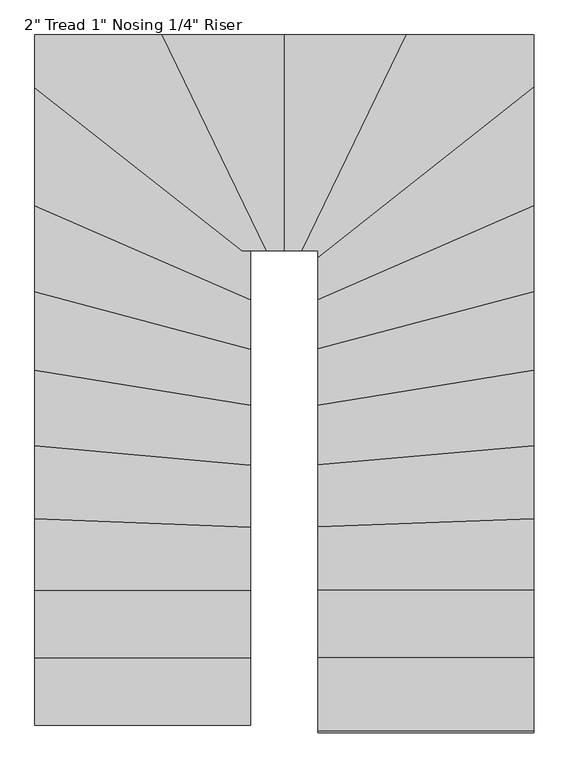
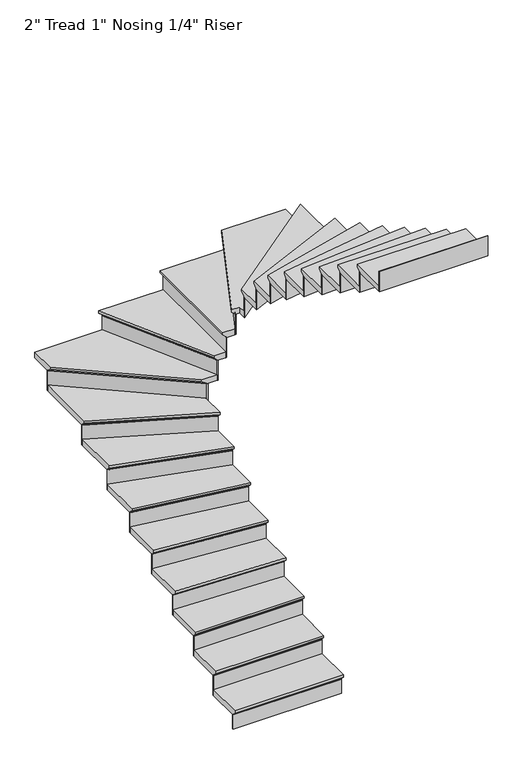
"""IFC4 building model written with IfcOpenShell, lengths in millimetres: stair flight geometry."""

from ifc_helpers import new_model, si_unit, origin, place, context, project, spatial, faceted_brep, source, transform, mapped, element, save


def stair_flight_d4b8cc4c(model_context):
    return source(origin(), model_context, "Body", "Brep", [
        faceted_brep([(-5047.1987704, -4554.2130548, 40388.7214286), (-5047.1987704, -4554.2130548, 40407.7714286), (-5940.8822214, -4554.2130548, 40407.7714286), (-5940.8822214, -4554.2130548, 40388.7214286), (-5047.1987704, -4528.8130548, 40363.3214286), (-5940.8822214, -4528.8130548, 40363.3214286), (-5047.1987704, -4249.4130548, 40407.7714286), (-5940.8822214, -4249.4130548, 40407.7714286), (-5940.8822214, -4528.8130548, 40356.9714286), (-5940.8822214, -4249.4130548, 40356.9714286), (-5047.1987704, -4249.4130548, 40356.9714286), (-5047.1987704, -4528.8130548, 40356.9714286)], [[[0, 1, 2, 3]], [[4, 0, 3, 5]], [[2, 1, 6, 7]], [[8, 9, 10, 11]], [[2, 7, 9, 8, 5, 3]], [[8, 11, 4, 5]], [[6, 1, 0, 4, 11, 10]], [[7, 6, 10, 9]]]),
        faceted_brep([(-5047.1987704, -4528.8130548, 40356.9714286), (-5047.1987704, -4528.8130548, 40233.6), (-5047.1987704, -4522.4630548, 40233.6), (-5047.1987704, -4522.4630548, 40356.9714286), (-5940.8822214, -4528.8130548, 40356.9714286), (-5940.8822214, -4522.4630548, 40356.9714286), (-5940.8822214, -4522.4630548, 40233.6), (-5940.8822214, -4528.8130548, 40233.6)], [[[0, 1, 2, 3]], [[4, 5, 6, 7]], [[1, 0, 4, 7]], [[2, 1, 7, 6]], [[3, 2, 6, 5]], [[0, 3, 5, 4]]]),
        faceted_brep([(-5047.1987704, -4249.4130548, 40531.1428571), (-5047.1987704, -4249.4130548, 40356.9714286), (-5047.1987704, -4243.0630548, 40356.9714286), (-5047.1987704, -4243.0630548, 40531.1428571), (-5940.8822214, -4249.4130548, 40531.1428571), (-5940.8822214, -4243.0630548, 40531.1428571), (-5940.8822214, -4243.0630548, 40356.9714286), (-5940.8822214, -4249.4130548, 40356.9714286)], [[[0, 1, 2, 3]], [[4, 5, 6, 7]], [[1, 0, 4, 7]], [[2, 1, 7, 6]], [[3, 2, 6, 5]], [[0, 3, 5, 4]]]),
        faceted_brep([(-5940.8822214, -4274.8130548, 40581.9428571), (-5047.1987704, -4274.8130548, 40581.9428571), (-5047.1987704, -3970.0130548, 40581.9428571), (-5940.8822214, -3970.0130548, 40581.9428571), (-5940.8822214, -4249.4130548, 40531.1428571), (-5940.8822214, -3970.0130548, 40531.1428571), (-5047.1987704, -3970.0130548, 40531.1428571), (-5047.1987704, -4249.4130548, 40531.1428571), (-5940.8822214, -4249.4130548, 40537.4928571), (-5940.8822214, -4274.8130548, 40562.8928571), (-5047.1987704, -4249.4130548, 40537.4928571), (-5047.1987704, -4274.8130548, 40562.8928571)], [[[0, 1, 2, 3]], [[4, 5, 6, 7]], [[0, 3, 5, 4, 8, 9]], [[4, 7, 10, 8]], [[2, 1, 11, 10, 7, 6]], [[3, 2, 6, 5]], [[11, 1, 0, 9]], [[10, 11, 9, 8]]]),
        faceted_brep([(-5047.1987704, -3970.0130548, 40705.3142857), (-5047.1987704, -3970.0130548, 40531.1428571), (-5047.1987704, -3963.6630548, 40531.1428571), (-5047.1987704, -3963.6630548, 40705.3142857), (-5940.8822214, -3970.0130548, 40705.3142857), (-5940.8822214, -3963.6630548, 40705.3142857), (-5940.8822214, -3963.6630548, 40531.1428571), (-5940.8822214, -3970.0130548, 40531.1428571)], [[[0, 1, 2, 3]], [[4, 5, 6, 7]], [[1, 0, 4, 7]], [[2, 1, 7, 6]], [[3, 2, 6, 5]], [[0, 3, 5, 4]]]),
        faceted_brep([(-5940.8822214, -3995.4130548, 40756.1142857), (-5047.1987704, -3995.4130548, 40756.1142857), (-5047.1987704, -3707.9036879, 40756.1142857), (-5940.8822214, -3673.2843203, 40756.1142857), (-5940.8822214, -3970.0130548, 40705.3142857), (-5940.8822214, -3673.2843203, 40705.3142857), (-5047.1987704, -3707.9036879, 40705.3142857), (-5047.1987704, -3970.0130548, 40705.3142857), (-5940.8822214, -3970.0130548, 40711.6642857), (-5940.8822214, -3995.4130548, 40737.0642857), (-5047.1987704, -3970.0130548, 40711.6642857), (-5047.1987704, -3995.4130548, 40737.0642857)], [[[0, 1, 2, 3]], [[4, 5, 6, 7]], [[0, 3, 5, 4, 8, 9]], [[4, 7, 10, 8]], [[2, 1, 11, 10, 7, 6]], [[3, 2, 6, 5]], [[11, 1, 0, 9]], [[10, 11, 9, 8]]]),
        faceted_brep([(-5047.1987704, -3707.9036879, 40879.4857143), (-5047.1987704, -3707.9036879, 40705.3142857), (-5047.1987704, -3701.5489252, 40705.3142857), (-5047.1987704, -3701.5489252, 40879.4857143), (-5940.8822214, -3673.2843203, 40879.4857143), (-5940.8822214, -3666.9295576, 40879.4857143), (-5940.8822214, -3666.9295576, 40705.3142857), (-5940.8822214, -3673.2843203, 40705.3142857)], [[[0, 1, 2, 3]], [[4, 5, 6, 7]], [[1, 0, 4, 7]], [[2, 1, 7, 6]], [[3, 2, 6, 5]], [[0, 3, 5, 4]]]),
        faceted_brep([(-5940.8822214, -3698.703371, 40930.2857143), (-5047.1987704, -3733.3227386, 40930.2857143), (-5047.1987704, -3451.3234819, 40930.2857143), (-5940.8822214, -3370.89733, 40930.2857143), (-5940.8822214, -3673.2843203, 40879.4857143), (-5940.8822214, -3370.89733, 40879.4857143), (-5047.1987704, -3451.3234819, 40879.4857143), (-5047.1987704, -3707.9036879, 40879.4857143), (-5940.8822214, -3673.2843203, 40885.8357143), (-5940.8822214, -3698.703371, 40911.2357143), (-5047.1987704, -3707.9036879, 40885.8357143), (-5047.1987704, -3733.3227386, 40911.2357143)], [[[0, 1, 2, 3]], [[4, 5, 6, 7]], [[0, 3, 5, 4, 8, 9]], [[4, 7, 10, 8]], [[2, 1, 11, 10, 7, 6]], [[3, 2, 6, 5]], [[11, 1, 0, 9]], [[10, 11, 9, 8]]]),
        faceted_brep([(-5047.1987704, -3451.3234819, 41053.6571429), (-5047.1987704, -3451.3234819, 40879.4857143), (-5047.1987704, -3444.9478197, 40879.4857143), (-5047.1987704, -3444.9478197, 41053.6571429), (-5940.8822214, -3370.89733, 41053.6571429), (-5940.8822214, -3364.5216678, 41053.6571429), (-5940.8822214, -3364.5216678, 40879.4857143), (-5940.8822214, -3370.89733, 40879.4857143)], [[[0, 1, 2, 3]], [[4, 5, 6, 7]], [[1, 0, 4, 7]], [[2, 1, 7, 6]], [[3, 2, 6, 5]], [[0, 3, 5, 4]]]),
        faceted_brep([(-5940.8822214, -3396.3999789, 41104.4571429), (-5047.1987704, -3476.8261308, 41104.4571429), (-5047.1987704, -3203.4301079, 41104.4571429), (-5940.8822214, -3059.5417727, 41104.4571429), (-5940.8822214, -3370.89733, 41053.6571429), (-5940.8822214, -3059.5417727, 41053.6571429), (-5047.1987704, -3203.4301079, 41053.6571429), (-5047.1987704, -3451.3234819, 41053.6571429), (-5940.8822214, -3370.89733, 41060.0071429), (-5940.8822214, -3396.3999789, 41085.4071429), (-5047.1987704, -3451.3234819, 41060.0071429), (-5047.1987704, -3476.8261308, 41085.4071429)], [[[0, 1, 2, 3]], [[4, 5, 6, 7]], [[0, 3, 5, 4, 8, 9]], [[4, 7, 10, 8]], [[2, 1, 11, 10, 7, 6]], [[3, 2, 6, 5]], [[11, 1, 0, 9]], [[10, 11, 9, 8]]]),
        faceted_brep([(-5047.1987704, -3203.4301079, 41227.8285714), (-5047.1987704, -3203.4301079, 41053.6571429), (-5047.1987704, -3196.9983292, 41053.6571429), (-5047.1987704, -3196.9983292, 41227.8285714), (-5940.8822214, -3059.5417727, 41227.8285714), (-5940.8822214, -3053.109994, 41227.8285714), (-5940.8822214, -3053.109994, 41053.6571429), (-5940.8822214, -3059.5417727, 41053.6571429)], [[[0, 1, 2, 3]], [[4, 5, 6, 7]], [[1, 0, 4, 7]], [[2, 1, 7, 6]], [[3, 2, 6, 5]], [[0, 3, 5, 4]]]),
        faceted_brep([(-5940.8822214, -3085.2688872, 41278.6285714), (-5047.1987704, -3229.1572224, 41278.6285714), (-5047.1987704, -2970.3553609, 41278.6285714), (-5940.8822214, -2732.7052783, 41278.6285714), (-5940.8822214, -3059.5417727, 41227.8285714), (-5940.8822214, -2732.7052783, 41227.8285714), (-5047.1987704, -2970.3553609, 41227.8285714), (-5047.1987704, -3203.4301079, 41227.8285714), (-5940.8822214, -3059.5417727, 41234.1785714), (-5940.8822214, -3085.2688872, 41259.5785714), (-5047.1987704, -3203.4301079, 41234.1785714), (-5047.1987704, -3229.1572224, 41259.5785714)], [[[0, 1, 2, 3]], [[4, 5, 6, 7]], [[0, 3, 5, 4, 8, 9]], [[4, 7, 10, 8]], [[2, 1, 11, 10, 7, 6]], [[3, 2, 6, 5]], [[11, 1, 0, 9]], [[10, 11, 9, 8]]]),
        faceted_brep([(-5047.1987704, -2970.3553609, 41402.0), (-5047.1987704, -2970.3553609, 41227.8285714), (-5047.1987704, -2963.7846771, 41227.8285714), (-5047.1987704, -2963.7846771, 41402.0), (-5940.8822214, -2732.7052783, 41402.0), (-5940.8822214, -2726.1345945, 41402.0), (-5940.8822214, -2726.1345945, 41227.8285714), (-5940.8822214, -2732.7052783, 41227.8285714)], [[[0, 1, 2, 3]], [[4, 5, 6, 7]], [[1, 0, 4, 7]], [[2, 1, 7, 6]], [[3, 2, 6, 5]], [[0, 3, 5, 4]]]),
        faceted_brep([(-5940.8822214, -2758.9880136, 41452.8), (-5047.1987704, -2996.6380961, 41452.8), (-5047.1987704, -2765.8050203, 41452.8), (-5940.8822214, -2375.5896532, 41452.8), (-5940.8822214, -2732.7052783, 41402.0), (-5940.8822214, -2375.5896532, 41402.0), (-5047.1987704, -2765.8050203, 41402.0), (-5047.1987704, -2970.3553609, 41402.0), (-5940.8822214, -2732.7052783, 41408.35), (-5940.8822214, -2758.9880136, 41433.75), (-5047.1987704, -2970.3553609, 41408.35), (-5047.1987704, -2996.6380961, 41433.75)], [[[0, 1, 2, 3]], [[4, 5, 6, 7]], [[0, 3, 5, 4, 8, 9]], [[4, 7, 10, 8]], [[2, 1, 11, 10, 7, 6]], [[3, 2, 6, 5]], [[11, 1, 0, 9]], [[10, 11, 9, 8]]]),
        faceted_brep([(-5047.1987704, -2765.8050203, 41576.1714286), (-5047.1987704, -2765.8050203, 41402.0), (-5047.1987704, -2758.8760908, 41402.0), (-5047.1987704, -2758.8760908, 41576.1714286), (-5940.8822214, -2375.5896532, 41576.1714286), (-5940.8822214, -2368.6607237, 41576.1714286), (-5940.8822214, -2368.6607237, 41402.0), (-5940.8822214, -2375.5896532, 41402.0)], [[[0, 1, 2, 3]], [[4, 5, 6, 7]], [[1, 0, 4, 7]], [[2, 1, 7, 6]], [[3, 2, 6, 5]], [[0, 3, 5, 4]]]),
        faceted_brep([(-5940.8822214, -2403.3053713, 41626.9714286), (-5047.1987704, -2793.5207384, 41626.9714286), (-5047.1987704, -2590.8424524, 41626.9714286), (-5040.8038639, -2590.8424524, 41626.9714286), (-5940.8822214, -1882.1944717, 41626.9714286), (-5940.8822214, -2375.5896532, 41576.1714286), (-5940.8822214, -1882.1944717, 41576.1714286), (-5040.8038639, -2590.8424524, 41576.1714286), (-5047.1987704, -2590.8424524, 41576.1714286), (-5047.1987704, -2765.8050203, 41576.1714286), (-5940.8822214, -2375.5896532, 41582.5214286), (-5940.8822214, -2403.3053713, 41607.9214286), (-5047.1987704, -2765.8050203, 41582.5214286), (-5047.1987704, -2793.5207384, 41607.9214286)], [[[0, 1, 2, 3, 4]], [[5, 6, 7, 8, 9]], [[0, 4, 6, 5, 10, 11]], [[5, 9, 12, 10]], [[2, 1, 13, 12, 9, 8]], [[4, 3, 7, 6]], [[13, 1, 0, 11]], [[12, 13, 11, 10]], [[3, 2, 8, 7]]]),
        faceted_brep([(-5040.8038639, -2590.8424524, 41750.3428571), (-5040.8038639, -2590.8424524, 41576.1714286), (-5030.5387554, -2590.8424524, 41576.1714286), (-5030.5387554, -2590.8424524, 41750.3428571), (-5940.8822214, -1882.1944717, 41750.3428571), (-5940.8822214, -1874.1125661, 41750.3428571), (-5940.8822214, -1874.1125661, 41576.1714286), (-5940.8822214, -1882.1944717, 41576.1714286)], [[[0, 1, 2, 3]], [[4, 5, 6, 7]], [[1, 0, 4, 7]], [[2, 1, 7, 6]], [[3, 2, 6, 5]], [[0, 3, 5, 4]]]),
        faceted_brep([(-5384.6489457, -1697.1590014, 41801.1428571), (-5940.8822214, -1697.1590014, 41801.1428571), (-5940.8822214, -1914.5220945, 41801.1428571), (-5081.8642978, -2590.8424524, 41801.1428571), (-4952.3566185, -2590.8424524, 41801.1428571), (-5940.8822214, -1697.1590014, 41750.3428571), (-5384.6489457, -1697.1590014, 41750.3428571), (-4952.3566185, -2590.8424524, 41750.3428571), (-5040.8038639, -2590.8424524, 41750.3428571), (-5940.8822214, -1882.1944717, 41750.3428571), (-5940.8822214, -1882.1944717, 41756.6928571), (-5940.8822214, -1914.5220945, 41782.0928571), (-5040.8038639, -2590.8424524, 41756.6928571), (-5081.8642978, -2590.8424524, 41782.0928571)], [[[0, 1, 2, 3, 4]], [[5, 6, 7, 8, 9]], [[1, 0, 6, 5]], [[2, 1, 5, 9, 10, 11]], [[9, 8, 12, 10]], [[4, 3, 13, 12, 8, 7]], [[0, 4, 7, 6]], [[13, 3, 2, 11]], [[12, 13, 11, 10]]]),
        faceted_brep([(-4952.3566185, -2590.8424524, 41924.5142857), (-4952.3566185, -2590.8424524, 41750.3428571), (-4945.3027294, -2590.8424524, 41750.3428571), (-4945.3027294, -2590.8424524, 41924.5142857), (-5384.6489457, -1697.1590014, 41924.5142857), (-5377.5950566, -1697.1590014, 41924.5142857), (-5377.5950566, -1697.1590014, 41750.3428571), (-5384.6489457, -1697.1590014, 41750.3428571)], [[[0, 1, 2, 3]], [[4, 5, 6, 7]], [[1, 0, 4, 7]], [[2, 1, 7, 6]], [[3, 2, 6, 5]], [[0, 3, 5, 4]]]),
        faceted_brep([(-5412.8645022, -1697.1590014, 41975.3142857), (-4980.5721749, -2590.8424524, 41975.3142857), (-4882.0987704, -2590.8424524, 41975.3142857), (-4882.0987706, -1697.1590014, 41975.3142857), (-5384.6489457, -1697.1590014, 41924.5142857), (-4882.0987706, -1697.1590014, 41924.5142857), (-4882.0987704, -2590.8424524, 41924.5142857), (-4952.3566185, -2590.8424524, 41924.5142857), (-5384.6489457, -1697.1590014, 41930.8642857), (-5412.8645022, -1697.1590014, 41956.2642857), (-4952.3566185, -2590.8424524, 41930.8642857), (-4980.5721749, -2590.8424524, 41956.2642857)], [[[0, 1, 2, 3]], [[4, 5, 6, 7]], [[0, 3, 5, 4, 8, 9]], [[4, 7, 10, 8]], [[3, 2, 6, 5]], [[11, 1, 0, 9]], [[10, 11, 9, 8]], [[2, 1, 11, 10, 7, 6]]]),
        faceted_brep([(-4882.0987704, -2590.8424524, 42098.6857143), (-4882.0987704, -2590.8424524, 41924.5142857), (-4875.7487704, -2590.8424524, 41924.5142857), (-4875.7487704, -2590.8424524, 42098.6857143), (-4882.0987706, -1697.1590014, 42098.6857143), (-4875.7487706, -1697.1590014, 42098.6857143), (-4875.7487706, -1697.1590014, 41924.5142857), (-4882.0987706, -1697.1590014, 41924.5142857)], [[[0, 1, 2, 3]], [[4, 5, 6, 7]], [[1, 0, 4, 7]], [[2, 1, 7, 6]], [[3, 2, 6, 5]], [[0, 3, 5, 4]]]),
        faceted_brep([(-4907.4987706, -1697.1590014, 42149.4857143), (-4907.4987704, -2590.8424524, 42149.4857143), (-4806.2098095, -2590.8424524, 42149.4857143), (-4373.9174828, -1697.1590014, 42149.4857143), (-4882.0987706, -1697.1590014, 42098.6857143), (-4373.9174828, -1697.1590014, 42098.6857143), (-4806.2098095, -2590.8424524, 42098.6857143), (-4882.0987704, -2590.8424524, 42098.6857143), (-4882.0987706, -1697.1590014, 42105.0357143), (-4907.4987706, -1697.1590014, 42130.4357143), (-4882.0987704, -2590.8424524, 42105.0357143), (-4907.4987704, -2590.8424524, 42130.4357143)], [[[0, 1, 2, 3]], [[4, 5, 6, 7]], [[0, 3, 5, 4, 8, 9]], [[4, 7, 10, 8]], [[2, 1, 11, 10, 7, 6]], [[3, 2, 6, 5]], [[11, 1, 0, 9]], [[10, 11, 9, 8]]]),
        faceted_brep([(-4806.2098095, -2590.8424524, 42272.8571429), (-4806.2098095, -2590.8424524, 42098.6857143), (-4799.1559204, -2590.8424524, 42098.6857143), (-4799.1559204, -2590.8424524, 42272.8571429), (-4373.9174828, -1697.1590014, 42272.8571429), (-4366.8635937, -1697.1590014, 42272.8571429), (-4366.8635937, -1697.1590014, 42098.6857143), (-4373.9174828, -1697.1590014, 42098.6857143)], [[[0, 1, 2, 3]], [[4, 5, 6, 7]], [[1, 0, 4, 7]], [[2, 1, 7, 6]], [[3, 2, 6, 5]], [[0, 3, 5, 4]]]),
        faceted_brep([(-3874.1153195, -1946.8497166, 42323.6571429), (-3874.1153195, -1697.1590014, 42323.6571429), (-4402.1330392, -1697.1590014, 42323.6571429), (-4834.4253659, -2590.8424524, 42323.6571429), (-4767.7987704, -2590.8424524, 42323.6571429), (-4767.7987704, -2650.4628721, 42323.6571429), (-3874.1153195, -1697.1590014, 42272.8571429), (-3874.1153195, -1946.8497166, 42272.8571429), (-4767.7987704, -2650.4628721, 42272.8571429), (-4767.7987704, -2590.8424524, 42272.8571429), (-4806.2098095, -2590.8424524, 42272.8571429), (-4373.9174828, -1697.1590014, 42272.8571429), (-4806.2098095, -2590.8424524, 42279.2071429), (-4373.9174828, -1697.1590014, 42279.2071429), (-4834.4253659, -2590.8424524, 42304.6071429), (-4402.1330392, -1697.1590014, 42304.6071429)], [[[0, 1, 2, 3, 4, 5]], [[6, 7, 8, 9, 10, 11]], [[1, 0, 7, 6]], [[11, 10, 12, 13]], [[4, 3, 14, 12, 10, 9]], [[5, 4, 9, 8]], [[0, 5, 8, 7]], [[14, 3, 2, 15]], [[12, 14, 15, 13]], [[2, 1, 6, 11, 13, 15]]]),
        faceted_brep([(-4767.7987704, -2650.4628721, 42447.0285714), (-4767.7987704, -2650.4628721, 42272.8571429), (-4767.7987704, -2658.5447778, 42272.8571429), (-4767.7987704, -2658.5447778, 42447.0285714), (-3874.1153195, -1946.8497166, 42447.0285714), (-3874.1153195, -1954.9316222, 42447.0285714), (-3874.1153195, -1954.9316222, 42272.8571429), (-3874.1153195, -1946.8497166, 42272.8571429)], [[[0, 1, 2, 3]], [[4, 5, 6, 7]], [[1, 0, 4, 7]], [[2, 1, 7, 6]], [[3, 2, 6, 5]], [[0, 3, 5, 4]]]),
        faceted_brep([(-3874.1153195, -1914.5220938, 42497.8285714), (-4767.7987704, -2618.1352494, 42497.8285714), (-4767.7987704, -2821.2364563, 42497.8285714), (-3874.1153195, -2431.0210889, 42497.8285714), (-3874.1153195, -1946.8497166, 42447.0285714), (-3874.1153195, -2431.0210889, 42447.0285714), (-4767.7987704, -2821.2364563, 42447.0285714), (-4767.7987704, -2650.4628721, 42447.0285714), (-3874.1153195, -1946.8497166, 42453.3785714), (-3874.1153195, -1914.5220938, 42478.7785714), (-4767.7987704, -2650.4628721, 42453.3785714), (-4767.7987704, -2618.1352494, 42478.7785714)], [[[0, 1, 2, 3]], [[4, 5, 6, 7]], [[0, 3, 5, 4, 8, 9]], [[4, 7, 10, 8]], [[2, 1, 11, 10, 7, 6]], [[3, 2, 6, 5]], [[11, 1, 0, 9]], [[10, 11, 9, 8]]]),
        faceted_brep([(-4767.7987704, -2821.2364563, 42621.2), (-4767.7987704, -2821.2364563, 42447.0285714), (-4767.7987704, -2828.1653858, 42447.0285714), (-4767.7987704, -2828.1653858, 42621.2), (-3874.1153195, -2431.0210889, 42621.2), (-3874.1153195, -2437.9500185, 42621.2), (-3874.1153195, -2437.9500185, 42447.0285714), (-3874.1153195, -2431.0210889, 42447.0285714)], [[[0, 1, 2, 3]], [[4, 5, 6, 7]], [[1, 0, 4, 7]], [[2, 1, 7, 6]], [[3, 2, 6, 5]], [[0, 3, 5, 4]]]),
        faceted_brep([(-3874.1153195, -2403.3053709, 42672.0), (-4767.7987704, -2793.5207382, 42672.0), (-4767.7987704, -3022.9208311, 42672.0), (-3874.1153195, -2785.2707484, 42672.0), (-3874.1153195, -2431.0210889, 42621.2), (-3874.1153195, -2785.2707484, 42621.2), (-4767.7987704, -3022.9208311, 42621.2), (-4767.7987704, -2821.2364563, 42621.2), (-3874.1153195, -2431.0210889, 42627.55), (-3874.1153195, -2403.3053709, 42652.95), (-4767.7987704, -2821.2364563, 42627.55), (-4767.7987704, -2793.5207382, 42652.95)], [[[0, 1, 2, 3]], [[4, 5, 6, 7]], [[0, 3, 5, 4, 8, 9]], [[4, 7, 10, 8]], [[2, 1, 11, 10, 7, 6]], [[3, 2, 6, 5]], [[11, 1, 0, 9]], [[10, 11, 9, 8]]]),
        faceted_brep([(-4767.7987704, -3022.9208311, 42795.3714286), (-4767.7987704, -3022.9208311, 42621.2), (-4767.7987704, -3029.4915149, 42621.2), (-4767.7987704, -3029.4915149, 42795.3714286), (-3874.1153195, -2785.2707484, 42795.3714286), (-3874.1153195, -2791.8414322, 42795.3714286), (-3874.1153195, -2791.8414322, 42621.2), (-3874.1153195, -2785.2707484, 42621.2)], [[[0, 1, 2, 3]], [[4, 5, 6, 7]], [[1, 0, 4, 7]], [[2, 1, 7, 6]], [[3, 2, 6, 5]], [[0, 3, 5, 4]]]),
        faceted_brep([(-3874.1153195, -2758.9880132, 42846.1714286), (-4767.7987704, -2996.6380959, 42846.1714286), (-4767.7987704, -3254.8843368, 42846.1714286), (-3874.1153195, -3110.9960015, 42846.1714286), (-3874.1153195, -2785.2707484, 42795.3714286), (-3874.1153195, -3110.9960015, 42795.3714286), (-4767.7987704, -3254.8843368, 42795.3714286), (-4767.7987704, -3022.9208311, 42795.3714286), (-3874.1153195, -2785.2707484, 42801.7214286), (-3874.1153195, -2758.9880132, 42827.1214286), (-4767.7987704, -3022.9208311, 42801.7214286), (-4767.7987704, -2996.6380959, 42827.1214286)], [[[0, 1, 2, 3]], [[4, 5, 6, 7]], [[0, 3, 5, 4, 8, 9]], [[4, 7, 10, 8]], [[2, 1, 11, 10, 7, 6]], [[3, 2, 6, 5]], [[11, 1, 0, 9]], [[10, 11, 9, 8]]]),
        faceted_brep([(-4767.7987704, -3254.8843368, 42969.5428571), (-4767.7987704, -3254.8843368, 42795.3714286), (-4767.7987704, -3261.3161154, 42795.3714286), (-4767.7987704, -3261.3161154, 42969.5428571), (-3874.1153195, -3110.9960015, 42969.5428571), (-3874.1153195, -3117.4277801, 42969.5428571), (-3874.1153195, -3117.4277801, 42795.3714286), (-3874.1153195, -3110.9960015, 42795.3714286)], [[[0, 1, 2, 3]], [[4, 5, 6, 7]], [[1, 0, 4, 7]], [[2, 1, 7, 6]], [[3, 2, 6, 5]], [[0, 3, 5, 4]]]),
        faceted_brep([(-3874.1153195, -3085.2688869, 43020.3428571), (-4767.7987704, -3229.1572222, 43020.3428571), (-4767.7987704, -3502.3287795, 43020.3428571), (-3874.1153195, -3421.9026274, 43020.3428571), (-3874.1153195, -3110.9960015, 42969.5428571), (-3874.1153195, -3421.9026274, 42969.5428571), (-4767.7987704, -3502.3287795, 42969.5428571), (-4767.7987704, -3254.8843368, 42969.5428571), (-3874.1153195, -3110.9960015, 42975.8928571), (-3874.1153195, -3085.2688869, 43001.2928571), (-4767.7987704, -3254.8843368, 42975.8928571), (-4767.7987704, -3229.1572222, 43001.2928571)], [[[0, 1, 2, 3]], [[4, 5, 6, 7]], [[0, 3, 5, 4, 8, 9]], [[4, 7, 10, 8]], [[2, 1, 11, 10, 7, 6]], [[3, 2, 6, 5]], [[11, 1, 0, 9]], [[10, 11, 9, 8]]]),
        faceted_brep([(-4767.7987704, -3502.3287795, 43143.7142857), (-4767.7987704, -3502.3287795, 42969.5428571), (-4767.7987704, -3508.7044417, 42969.5428571), (-4767.7987704, -3508.7044417, 43143.7142857), (-3874.1153195, -3421.9026274, 43143.7142857), (-3874.1153195, -3428.2782897, 43143.7142857), (-3874.1153195, -3428.2782897, 42969.5428571), (-3874.1153195, -3421.9026274, 42969.5428571)], [[[0, 1, 2, 3]], [[4, 5, 6, 7]], [[1, 0, 4, 7]], [[2, 1, 7, 6]], [[3, 2, 6, 5]], [[0, 3, 5, 4]]]),
        faceted_brep([(-3874.1153195, -3396.3999786, 43194.5142857), (-4767.7987704, -3476.8261306, 43194.5142857), (-4767.7987704, -3758.7417891, 43194.5142857), (-3874.1153195, -3724.1224215, 43194.5142857), (-3874.1153195, -3421.9026274, 43143.7142857), (-3874.1153195, -3724.1224215, 43143.7142857), (-4767.7987704, -3758.7417891, 43143.7142857), (-4767.7987704, -3502.3287795, 43143.7142857), (-3874.1153195, -3421.9026274, 43150.0642857), (-3874.1153195, -3396.3999786, 43175.4642857), (-4767.7987704, -3502.3287795, 43150.0642857), (-4767.7987704, -3476.8261306, 43175.4642857)], [[[0, 1, 2, 3]], [[4, 5, 6, 7]], [[0, 3, 5, 4, 8, 9]], [[4, 7, 10, 8]], [[2, 1, 11, 10, 7, 6]], [[3, 2, 6, 5]], [[11, 1, 0, 9]], [[10, 11, 9, 8]]]),
        faceted_brep([(-4767.7987704, -3758.7417891, 43317.8857143), (-4767.7987704, -3758.7417891, 43143.7142857), (-4767.7987704, -3765.0965518, 43143.7142857), (-4767.7987704, -3765.0965518, 43317.8857143), (-3874.1153195, -3724.1224215, 43317.8857143), (-3874.1153195, -3730.4771842, 43317.8857143), (-3874.1153195, -3730.4771842, 43143.7142857), (-3874.1153195, -3724.1224215, 43143.7142857)], [[[0, 1, 2, 3]], [[4, 5, 6, 7]], [[1, 0, 4, 7]], [[2, 1, 7, 6]], [[3, 2, 6, 5]], [[0, 3, 5, 4]]]),
        faceted_brep([(-3874.1153195, -3698.7033708, 43368.6857143), (-4767.7987704, -3733.3227384, 43368.6857143), (-4767.7987704, -4020.8130546, 43368.6857143), (-3874.1153195, -4020.8130546, 43368.6857143), (-3874.1153195, -3724.1224215, 43317.8857143), (-3874.1153195, -4020.8130546, 43317.8857143), (-4767.7987704, -4020.8130546, 43317.8857143), (-4767.7987704, -3758.7417891, 43317.8857143), (-3874.1153195, -3724.1224215, 43324.2357143), (-3874.1153195, -3698.7033708, 43349.6357143), (-4767.7987704, -3758.7417891, 43324.2357143), (-4767.7987704, -3733.3227384, 43349.6357143)], [[[0, 1, 2, 3]], [[4, 5, 6, 7]], [[0, 3, 5, 4, 8, 9]], [[4, 7, 10, 8]], [[2, 1, 11, 10, 7, 6]], [[3, 2, 6, 5]], [[11, 1, 0, 9]], [[10, 11, 9, 8]]]),
        faceted_brep([(-4767.7987704, -4020.8130546, 43492.0571429), (-4767.7987704, -4020.8130546, 43317.8857143), (-4767.7987704, -4027.1630546, 43317.8857143), (-4767.7987704, -4027.1630546, 43492.0571429), (-3874.1153195, -4020.8130546, 43492.0571429), (-3874.1153195, -4027.1630546, 43492.0571429), (-3874.1153195, -4027.1630546, 43317.8857143), (-3874.1153195, -4020.8130546, 43317.8857143)], [[[0, 1, 2, 3]], [[4, 5, 6, 7]], [[1, 0, 4, 7]], [[2, 1, 7, 6]], [[3, 2, 6, 5]], [[0, 3, 5, 4]]]),
        faceted_brep([(-3874.1153195, -3995.4130546, 43542.8571429), (-4767.7987704, -3995.4130546, 43542.8571429), (-4767.7987704, -4300.2130546, 43542.8571429), (-3874.1153195, -4300.2130546, 43542.8571429), (-3874.1153195, -4020.8130546, 43492.0571429), (-3874.1153195, -4300.2130546, 43492.0571429), (-4767.7987704, -4300.2130546, 43492.0571429), (-4767.7987704, -4020.8130546, 43492.0571429), (-3874.1153195, -4020.8130546, 43498.4071429), (-3874.1153195, -3995.4130546, 43523.8071429), (-4767.7987704, -4020.8130546, 43498.4071429), (-4767.7987704, -3995.4130546, 43523.8071429)], [[[0, 1, 2, 3]], [[4, 5, 6, 7]], [[0, 3, 5, 4, 8, 9]], [[4, 7, 10, 8]], [[2, 1, 11, 10, 7, 6]], [[3, 2, 6, 5]], [[11, 1, 0, 9]], [[10, 11, 9, 8]]]),
        faceted_brep([(-4767.7987704, -4300.2130546, 43666.2285714), (-4767.7987704, -4300.2130546, 43492.0571429), (-4767.7987704, -4306.5630546, 43492.0571429), (-4767.7987704, -4306.5630546, 43666.2285714), (-3874.1153195, -4300.2130546, 43666.2285714), (-3874.1153195, -4306.5630546, 43666.2285714), (-3874.1153195, -4306.5630546, 43492.0571429), (-3874.1153195, -4300.2130546, 43492.0571429)], [[[0, 1, 2, 3]], [[4, 5, 6, 7]], [[1, 0, 4, 7]], [[2, 1, 7, 6]], [[3, 2, 6, 5]], [[0, 3, 5, 4]]]),
        faceted_brep([(-4767.7987704, -4579.6130546, 43840.4), (-4767.7987704, -4579.6130546, 43666.2285714), (-4767.7987704, -4585.9630546, 43666.2285714), (-4767.7987704, -4585.9630546, 43840.4), (-3874.1153195, -4579.6130546, 43840.4), (-3874.1153195, -4585.9630546, 43840.4), (-3874.1153195, -4585.9630546, 43666.2285714), (-3874.1153195, -4579.6130546, 43666.2285714)], [[[0, 1, 2, 3]], [[4, 5, 6, 7]], [[1, 0, 4, 7]], [[2, 1, 7, 6]], [[3, 2, 6, 5]], [[0, 3, 5, 4]]]),
        faceted_brep([(-3874.1153195, -4274.8130546, 43717.0285714), (-4767.7987704, -4274.8130546, 43717.0285714), (-4767.7987704, -4579.6130546, 43717.0285714), (-3874.1153195, -4579.6130546, 43717.0285714), (-3874.1153195, -4300.2130546, 43666.2285714), (-3874.1153195, -4579.6130546, 43666.2285714), (-4767.7987704, -4579.6130546, 43666.2285714), (-4767.7987704, -4300.2130546, 43666.2285714), (-3874.1153195, -4300.2130546, 43672.5785714), (-3874.1153195, -4274.8130546, 43697.9785714), (-4767.7987704, -4300.2130546, 43672.5785714), (-4767.7987704, -4274.8130546, 43697.9785714)], [[[0, 1, 2, 3]], [[4, 5, 6, 7]], [[0, 3, 5, 4, 8, 9]], [[4, 7, 10, 8]], [[2, 1, 11, 10, 7, 6]], [[3, 2, 6, 5]], [[11, 1, 0, 9]], [[10, 11, 9, 8]]]),
    ])


if __name__ == "__main__":
    model = new_model("IFC4")
    model_context = context("Model", 3, world=origin())
    ifc_project = project(units=[si_unit("LENGTHUNIT", "METRE", prefix="MILLI")], contexts=[model_context])
    site = spatial("IfcSite", under=ifc_project)
    building = spatial("IfcBuilding", under=site)
    placement = place(None, origin())
    stair_flight_shape = stair_flight_d4b8cc4c(model_context)
    element("IfcStairFlight", 1, ObjectType="2\" Tread 1\" Nosing 1/4\" Riser", at=placement, inside=building, context=model_context, shape_type="MappedRepresentation", body=[
        mapped(stair_flight_shape, transform((0.0, 0.0, 0.0), x_axis=(1.0, 0.0, 0.0), y_axis=(0.0, 1.0, 0.0), z_axis=(0.0, 0.0, 1.0))),
    ])
    save(model, "model.ifc")

# Revit data of these elements
# Element 1 (IfcStairFlight, "2\" Tread 1\" Nosing 1/4\" Riser")
#   Materials on its faces: "Tile, Porcelain, 4in"
# Materials
#   "Tile, Porcelain, 4in": class "Generic", colour RGB 89 87 158, transparency 0, Description = "Porcelain tile, 4\", white", Cost = 0
